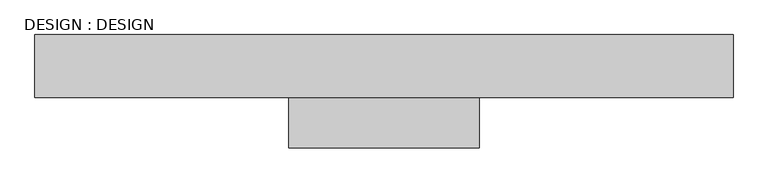
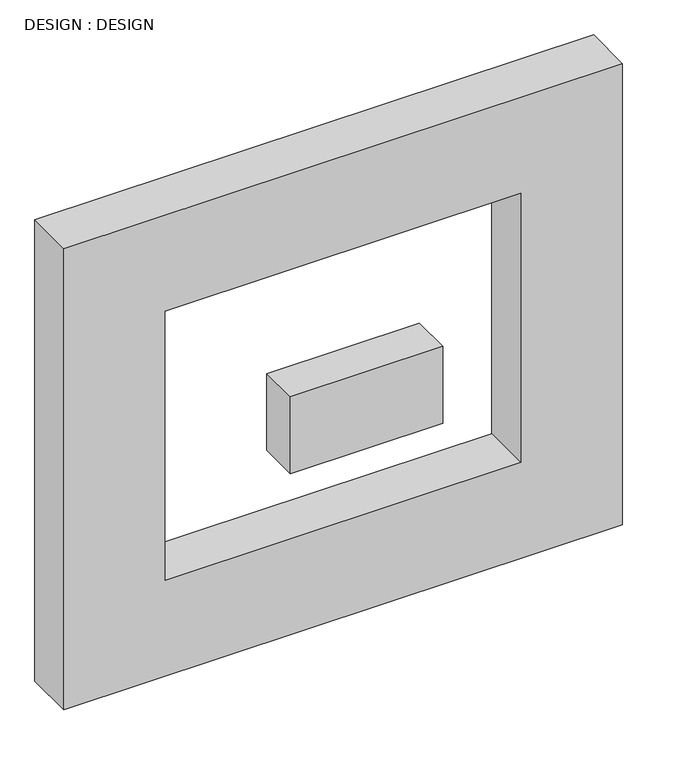
"""IFC4 building model written with IfcOpenShell, lengths in millimetres: proxy geometry, DESIGN : DESIGN."""

from ifc_helpers import new_model, si_unit, frame, origin, place, context, project, spatial, polyline, outline, extrude, source, transform, mapped, element, save


def design_design_48f371e7(model_context):
    return source(origin(), model_context, "Body", "SweptSolid", [
        extrude(outline(polyline([(-515.564062, -8072.6621669), (-896.564062, -8072.6621669), (-896.564062, -7971.0621669), (-515.564062, -7971.0621669), (-515.564062, -8072.6621669)])), frame((0.0, 0.0, 508.0), z_axis=(0.0, 0.0, 1.0), x_axis=(1.0, 0.0, 0.0)), (0.0, 0.0, 1.0), 203.2),
        extrude(outline(polyline([(0.0, -7.564062), (1219.2, -7.564062), (1219.2, -1404.564062), (0.0, -1404.564062), (0.0, -7.564062)]), holes=[polyline([(965.2, -261.564062), (254.0, -261.564062), (254.0, -1150.564062), (965.2, -1150.564062), (965.2, -261.564062)])]), frame((0.0, -7971.0621669, 0.0), z_axis=(0.0, 1.0, 0.0), x_axis=(0.0, 0.0, 1.0)), (0.0, 0.0, 1.0), 125.4479032),
    ])


if __name__ == "__main__":
    model = new_model("IFC4")
    model_context = context("Model", 3, world=origin())
    ifc_project = project(units=[si_unit("LENGTHUNIT", "METRE", prefix="MILLI")], contexts=[model_context])
    site = spatial("IfcSite", under=ifc_project)
    building = spatial("IfcBuilding", under=site)
    placement = place(None, origin())
    design_design_shape = design_design_48f371e7(model_context)
    element("IfcBuildingElementProxy", 1, Name="DESIGN : DESIGN", ObjectType="DESIGN : DESIGN", at=placement, inside=building, context=model_context, shape_type="MappedRepresentation", body=[
        mapped(design_design_shape, transform((0.0, 0.0, 0.0), x_axis=(1.0, 0.0, 0.0), y_axis=(0.0, 1.0, 0.0), z_axis=(0.0, 0.0, 1.0))),
    ])
    save(model, "model.ifc")

# Revit data of these elements
# Element 1 (IfcBuildingElementProxy, "DESIGN : DESIGN")
#   Materials on its faces: "DINING ROOM WALL"
# Materials
#   "DINING ROOM WALL": class "Generic", colour RGB 120 120 120, transparency 0, Cost = 0
